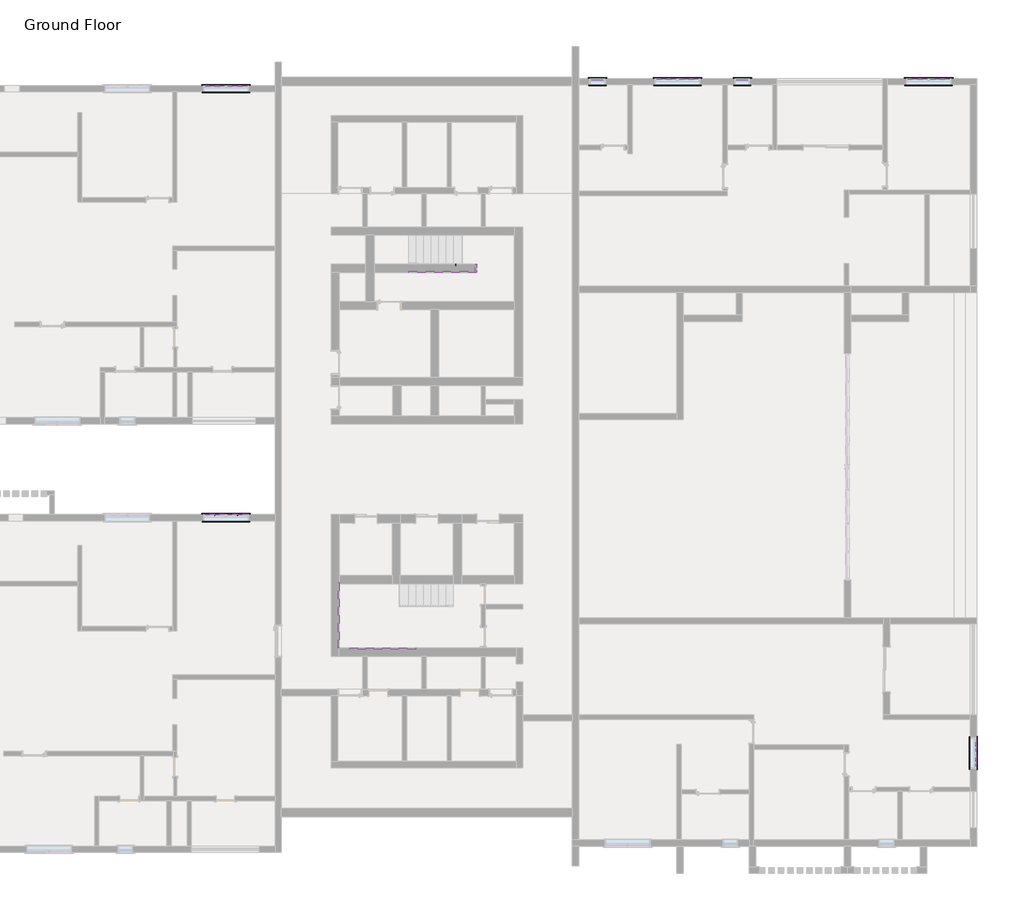
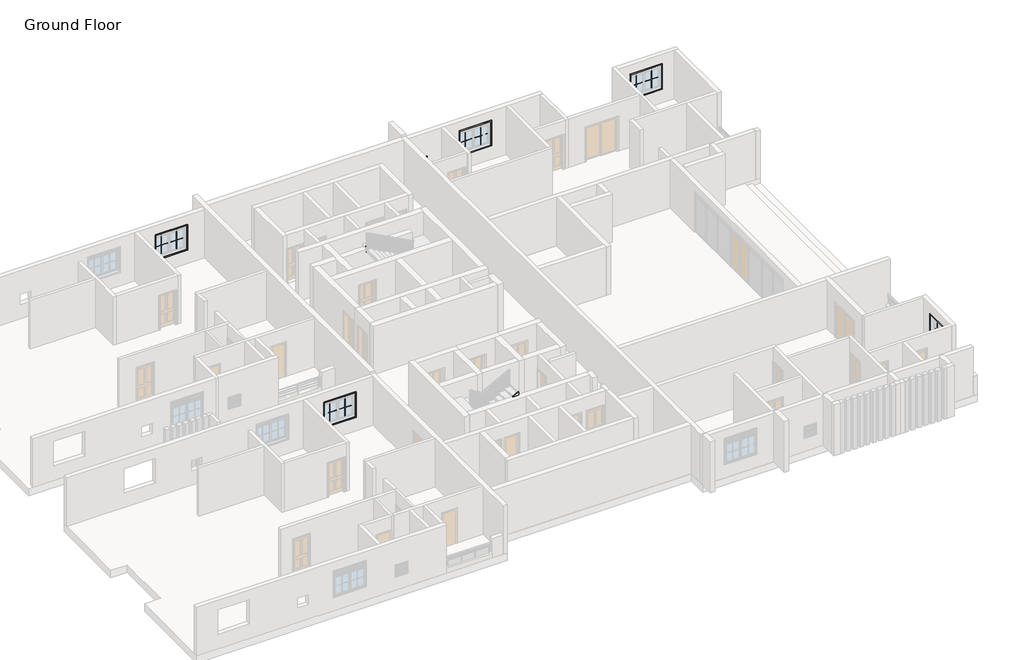
# One storey, part 9 of 9: 38 proxies, 6 members.
"""IFC4 building model written with IfcOpenShell, lengths in millimetres."""

from ifc_helpers import new_model, si_unit, frame, origin, place, context, project, spatial, polyline, outline, extrude, transform, mapped, element, save
from components import muntin_pattern_2x2_muntin_pattern_2x2_dc2504c2, muntin_pattern_2x2_muntin_pattern_2x2_0aa094e9, muntin_pattern_2x2_muntin_pattern_2x2_f17ebf58, muntin_pattern_2x2_muntin_pattern_2x2_cfeb24ad, muntin_pattern_2x2_muntin_pattern_2x2_4dfeb3f3, muntin_pattern_2x2_muntin_pattern_2x2_e852a7e4, muntin_pattern_2x2_muntin_pattern_2x2_3df65231, trim_window_exterior_flat_with_sill_c22f0c79, trim_window_exterior_flat_with_sill_858dc10d, trim_window_exterior_flat_with_sill_92b9b949, trim_window_interior_flat_picture_frame_d1f4d6ef, trim_window_interior_flat_picture_frame_3927330c, trim_window_interior_flat_picture_frame_3bb882cf

model = new_model("IFC4")

# Units and contexts
model_context = context("Model", 3, world=origin())
ifc_project = project(units=[si_unit("LENGTHUNIT", "METRE", prefix="MILLI")], contexts=[model_context])

# Site, building, storey
site = spatial("IfcSite", under=ifc_project)
building = spatial("IfcBuilding", under=site)
storey = spatial("IfcBuildingStorey", under=building, Name="Ground Floor", Elevation=0.0)

# Proxies
placement = place(None, origin())
muntin_pattern_2x2_muntin_pattern_2x2_shape = muntin_pattern_2x2_muntin_pattern_2x2_dc2504c2(model_context)
element("IfcBuildingElementProxy", 1, Name="Muntin Pattern_2x2 : Muntin Pattern_2x2", ObjectType="Muntin Pattern_2x2 : Muntin Pattern_2x2", at=placement, inside=storey, context=model_context, shape_type="MappedRepresentation", body=[
    mapped(muntin_pattern_2x2_muntin_pattern_2x2_shape, transform((1344.6421318, 11632.309892, 984.25), x_axis=(1.0, 0.0, 0.0), y_axis=(0.0, 1.0, 0.0), z_axis=(0.0, 0.0, 1.0))),
])
element("IfcBuildingElementProxy", 2, Name="Muntin Pattern_2x2 : Muntin Pattern_2x2", ObjectType="Muntin Pattern_2x2 : Muntin Pattern_2x2", at=placement, inside=storey, context=model_context, shape_type="MappedRepresentation", body=[
    mapped(muntin_pattern_2x2_muntin_pattern_2x2_shape, transform((1344.6421318, 28955.109892, 984.25), x_axis=(1.0, 0.0, 0.0), y_axis=(0.0, 1.0, 0.0), z_axis=(0.0, 0.0, 1.0))),
])
element("IfcBuildingElementProxy", 3, Name="Muntin Pattern_2x2 : Muntin Pattern_2x2", ObjectType="Muntin Pattern_2x2 : Muntin Pattern_2x2", at=placement, inside=storey, context=model_context, shape_type="MappedRepresentation", body=[
    mapped(muntin_pattern_2x2_muntin_pattern_2x2_shape, transform((19556.4421318, 29234.509892, 984.25), x_axis=(1.0, 0.0, 0.0), y_axis=(0.0, 1.0, 0.0), z_axis=(0.0, 0.0, 1.0))),
])
element("IfcBuildingElementProxy", 4, Name="Muntin Pattern_2x2 : Muntin Pattern_2x2", ObjectType="Muntin Pattern_2x2 : Muntin Pattern_2x2", at=placement, inside=storey, context=model_context, shape_type="MappedRepresentation", body=[
    mapped(muntin_pattern_2x2_muntin_pattern_2x2_shape, transform((29691.0421318, 29234.509892, 984.25), x_axis=(1.0, 0.0, 0.0), y_axis=(0.0, 1.0, 0.0), z_axis=(0.0, 0.0, 1.0))),
])
muntin_pattern_2x2_muntin_pattern_2x2_2_shape = muntin_pattern_2x2_muntin_pattern_2x2_0aa094e9(model_context)
element("IfcBuildingElementProxy", 5, Name="Muntin Pattern_2x2 : Muntin Pattern_2x2", ObjectType="Muntin Pattern_2x2 : Muntin Pattern_2x2", at=placement, inside=storey, context=model_context, shape_type="MappedRepresentation", body=[
    mapped(muntin_pattern_2x2_muntin_pattern_2x2_2_shape, transform((2255.8671318, 11632.309892, 984.25), x_axis=(-1.0, 0.0, 0.0), y_axis=(0.0, -1.0, 0.0), z_axis=(0.0, 0.0, 1.0))),
])
element("IfcBuildingElementProxy", 6, Name="Muntin Pattern_2x2 : Muntin Pattern_2x2", ObjectType="Muntin Pattern_2x2 : Muntin Pattern_2x2", at=placement, inside=storey, context=model_context, shape_type="MappedRepresentation", body=[
    mapped(muntin_pattern_2x2_muntin_pattern_2x2_2_shape, transform((2255.8671318, 28955.109892, 984.25), x_axis=(-1.0, 0.0, 0.0), y_axis=(0.0, -1.0, 0.0), z_axis=(0.0, 0.0, 1.0))),
])
element("IfcBuildingElementProxy", 7, Name="Muntin Pattern_2x2 : Muntin Pattern_2x2", ObjectType="Muntin Pattern_2x2 : Muntin Pattern_2x2", at=placement, inside=storey, context=model_context, shape_type="MappedRepresentation", body=[
    mapped(muntin_pattern_2x2_muntin_pattern_2x2_2_shape, transform((20467.6671318, 29234.509892, 984.25), x_axis=(-1.0, 0.0, 0.0), y_axis=(0.0, -1.0, 0.0), z_axis=(0.0, 0.0, 1.0))),
])
element("IfcBuildingElementProxy", 8, Name="Muntin Pattern_2x2 : Muntin Pattern_2x2", ObjectType="Muntin Pattern_2x2 : Muntin Pattern_2x2", at=placement, inside=storey, context=model_context, shape_type="MappedRepresentation", body=[
    mapped(muntin_pattern_2x2_muntin_pattern_2x2_2_shape, transform((30602.2671318, 29234.509892, 984.25), x_axis=(-1.0, 0.0, 0.0), y_axis=(0.0, -1.0, 0.0), z_axis=(0.0, 0.0, 1.0))),
])
muntin_pattern_2x2_muntin_pattern_2x2_3_shape = muntin_pattern_2x2_muntin_pattern_2x2_f17ebf58(model_context)
element("IfcBuildingElementProxy", 9, Name="Muntin Pattern_2x2 : Muntin Pattern_2x2", ObjectType="Muntin Pattern_2x2 : Muntin Pattern_2x2", at=placement, inside=storey, context=model_context, shape_type="MappedRepresentation", body=[
    mapped(muntin_pattern_2x2_muntin_pattern_2x2_3_shape, transform((2255.8671318, 11632.309892, 2203.45), x_axis=(-1.0, 0.0, 0.0), y_axis=(0.0, -1.0, 0.0), z_axis=(0.0, 0.0, 1.0))),
])
element("IfcBuildingElementProxy", 10, Name="Muntin Pattern_2x2 : Muntin Pattern_2x2", ObjectType="Muntin Pattern_2x2 : Muntin Pattern_2x2", at=placement, inside=storey, context=model_context, shape_type="MappedRepresentation", body=[
    mapped(muntin_pattern_2x2_muntin_pattern_2x2_3_shape, transform((1344.6421318, 11632.309892, 2203.45), x_axis=(-1.0, 0.0, 0.0), y_axis=(0.0, -1.0, 0.0), z_axis=(0.0, 0.0, 1.0))),
])
element("IfcBuildingElementProxy", 11, Name="Muntin Pattern_2x2 : Muntin Pattern_2x2", ObjectType="Muntin Pattern_2x2 : Muntin Pattern_2x2", at=placement, inside=storey, context=model_context, shape_type="MappedRepresentation", body=[
    mapped(muntin_pattern_2x2_muntin_pattern_2x2_3_shape, transform((2255.8671318, 28955.109892, 2203.45), x_axis=(-1.0, 0.0, 0.0), y_axis=(0.0, -1.0, 0.0), z_axis=(0.0, 0.0, 1.0))),
])
element("IfcBuildingElementProxy", 12, Name="Muntin Pattern_2x2 : Muntin Pattern_2x2", ObjectType="Muntin Pattern_2x2 : Muntin Pattern_2x2", at=placement, inside=storey, context=model_context, shape_type="MappedRepresentation", body=[
    mapped(muntin_pattern_2x2_muntin_pattern_2x2_3_shape, transform((1344.6421318, 28955.109892, 2203.45), x_axis=(-1.0, 0.0, 0.0), y_axis=(0.0, -1.0, 0.0), z_axis=(0.0, 0.0, 1.0))),
])
element("IfcBuildingElementProxy", 13, Name="Muntin Pattern_2x2 : Muntin Pattern_2x2", ObjectType="Muntin Pattern_2x2 : Muntin Pattern_2x2", at=placement, inside=storey, context=model_context, shape_type="MappedRepresentation", body=[
    mapped(muntin_pattern_2x2_muntin_pattern_2x2_3_shape, transform((20467.6671318, 29234.509892, 2203.45), x_axis=(-1.0, 0.0, 0.0), y_axis=(0.0, -1.0, 0.0), z_axis=(0.0, 0.0, 1.0))),
])
element("IfcBuildingElementProxy", 14, Name="Muntin Pattern_2x2 : Muntin Pattern_2x2", ObjectType="Muntin Pattern_2x2 : Muntin Pattern_2x2", at=placement, inside=storey, context=model_context, shape_type="MappedRepresentation", body=[
    mapped(muntin_pattern_2x2_muntin_pattern_2x2_3_shape, transform((19556.4421318, 29234.509892, 2203.45), x_axis=(-1.0, 0.0, 0.0), y_axis=(0.0, -1.0, 0.0), z_axis=(0.0, 0.0, 1.0))),
])
element("IfcBuildingElementProxy", 15, Name="Muntin Pattern_2x2 : Muntin Pattern_2x2", ObjectType="Muntin Pattern_2x2 : Muntin Pattern_2x2", at=placement, inside=storey, context=model_context, shape_type="MappedRepresentation", body=[
    mapped(muntin_pattern_2x2_muntin_pattern_2x2_3_shape, transform((30602.2671318, 29234.509892, 2203.45), x_axis=(-1.0, 0.0, 0.0), y_axis=(0.0, -1.0, 0.0), z_axis=(0.0, 0.0, 1.0))),
])
element("IfcBuildingElementProxy", 16, Name="Muntin Pattern_2x2 : Muntin Pattern_2x2", ObjectType="Muntin Pattern_2x2 : Muntin Pattern_2x2", at=placement, inside=storey, context=model_context, shape_type="MappedRepresentation", body=[
    mapped(muntin_pattern_2x2_muntin_pattern_2x2_3_shape, transform((29691.0421318, 29234.509892, 2203.45), x_axis=(-1.0, 0.0, 0.0), y_axis=(0.0, -1.0, 0.0), z_axis=(0.0, 0.0, 1.0))),
])
muntin_pattern_2x2_muntin_pattern_2x2_4_shape = muntin_pattern_2x2_muntin_pattern_2x2_cfeb24ad(model_context)
element("IfcBuildingElementProxy", 17, Name="Muntin Pattern_2x2 : Muntin Pattern_2x2", ObjectType="Muntin Pattern_2x2 : Muntin Pattern_2x2", at=placement, inside=storey, context=model_context, shape_type="MappedRepresentation", body=[
    mapped(muntin_pattern_2x2_muntin_pattern_2x2_4_shape, transform((22628.2546318, 29209.109892, 1241.425), x_axis=(1.0, 0.0, 0.0), y_axis=(0.0, 1.0, 0.0), z_axis=(0.0, 0.0, 1.0))),
])
element("IfcBuildingElementProxy", 18, Name="Muntin Pattern_2x2 : Muntin Pattern_2x2", ObjectType="Muntin Pattern_2x2 : Muntin Pattern_2x2", at=placement, inside=storey, context=model_context, shape_type="MappedRepresentation", body=[
    mapped(muntin_pattern_2x2_muntin_pattern_2x2_4_shape, transform((22628.2546318, 29164.659892, 990.6), x_axis=(1.0, 0.0, 0.0), y_axis=(0.0, 1.0, 0.0), z_axis=(0.0, 0.0, 1.0))),
])
element("IfcBuildingElementProxy", 19, Name="Muntin Pattern_2x2 : Muntin Pattern_2x2", ObjectType="Muntin Pattern_2x2 : Muntin Pattern_2x2", at=placement, inside=storey, context=model_context, shape_type="MappedRepresentation", body=[
    mapped(muntin_pattern_2x2_muntin_pattern_2x2_4_shape, transform((16786.2546318, 29209.109892, 1241.425), x_axis=(1.0, 0.0, 0.0), y_axis=(0.0, 1.0, 0.0), z_axis=(0.0, 0.0, 1.0))),
])
element("IfcBuildingElementProxy", 20, Name="Muntin Pattern_2x2 : Muntin Pattern_2x2", ObjectType="Muntin Pattern_2x2 : Muntin Pattern_2x2", at=placement, inside=storey, context=model_context, shape_type="MappedRepresentation", body=[
    mapped(muntin_pattern_2x2_muntin_pattern_2x2_4_shape, transform((16786.2546318, 29164.659892, 990.6), x_axis=(1.0, 0.0, 0.0), y_axis=(0.0, 1.0, 0.0), z_axis=(0.0, 0.0, 1.0))),
])
muntin_pattern_2x2_muntin_pattern_2x2_5_shape = muntin_pattern_2x2_muntin_pattern_2x2_4dfeb3f3(model_context)
element("IfcBuildingElementProxy", 21, Name="Muntin Pattern_2x2 : Muntin Pattern_2x2", ObjectType="Muntin Pattern_2x2 : Muntin Pattern_2x2", at=placement, inside=storey, context=model_context, shape_type="MappedRepresentation", body=[
    mapped(muntin_pattern_2x2_muntin_pattern_2x2_5_shape, transform((32067.5296318, 2318.447392, 984.25), x_axis=(0.0, -1.0, 0.0), y_axis=(1.0, 0.0, 0.0), z_axis=(0.0, 0.0, 1.0))),
])
muntin_pattern_2x2_muntin_pattern_2x2_6_shape = muntin_pattern_2x2_muntin_pattern_2x2_e852a7e4(model_context)
element("IfcBuildingElementProxy", 22, Name="Muntin Pattern_2x2 : Muntin Pattern_2x2", ObjectType="Muntin Pattern_2x2 : Muntin Pattern_2x2", at=placement, inside=storey, context=model_context, shape_type="MappedRepresentation", body=[
    mapped(muntin_pattern_2x2_muntin_pattern_2x2_6_shape, transform((32067.5296318, 1712.022392, 984.25), x_axis=(0.0, 1.0, 0.0), y_axis=(-1.0, 0.0, 0.0), z_axis=(0.0, 0.0, 1.0))),
])
muntin_pattern_2x2_muntin_pattern_2x2_7_shape = muntin_pattern_2x2_muntin_pattern_2x2_3df65231(model_context)
element("IfcBuildingElementProxy", 23, Name="Muntin Pattern_2x2 : Muntin Pattern_2x2", ObjectType="Muntin Pattern_2x2 : Muntin Pattern_2x2", at=placement, inside=storey, context=model_context, shape_type="MappedRepresentation", body=[
    mapped(muntin_pattern_2x2_muntin_pattern_2x2_7_shape, transform((32067.5296318, 1712.022392, 2203.45), x_axis=(0.0, 1.0, 0.0), y_axis=(-1.0, 0.0, 0.0), z_axis=(0.0, 0.0, 1.0))),
])
element("IfcBuildingElementProxy", 24, Name="Muntin Pattern_2x2 : Muntin Pattern_2x2", ObjectType="Muntin Pattern_2x2 : Muntin Pattern_2x2", at=placement, inside=storey, context=model_context, shape_type="MappedRepresentation", body=[
    mapped(muntin_pattern_2x2_muntin_pattern_2x2_7_shape, transform((32067.5296318, 2318.447392, 2203.45), x_axis=(0.0, 1.0, 0.0), y_axis=(-1.0, 0.0, 0.0), z_axis=(0.0, 0.0, 1.0))),
])
trim_window_exterior_flat_with_sill_shape = trim_window_exterior_flat_with_sill_c22f0c79(model_context)
element("IfcBuildingElementProxy", 25, Name="Trim-Window-Exterior-Flat : with Sill", ObjectType="Trim-Window-Exterior-Flat : with Sill", at=placement, inside=storey, context=model_context, shape_type="MappedRepresentation", body=[
    mapped(trim_window_exterior_flat_with_sill_shape, transform((1800.2546318, 11641.834892, 2438.4), x_axis=(-1.0, 0.0, 0.0), y_axis=(0.0, 0.0, 1.0), z_axis=(0.0, 1.0, 0.0))),
])
element("IfcBuildingElementProxy", 26, Name="Trim-Window-Exterior-Flat : with Sill", ObjectType="Trim-Window-Exterior-Flat : with Sill", at=placement, inside=storey, context=model_context, shape_type="MappedRepresentation", body=[
    mapped(trim_window_exterior_flat_with_sill_shape, transform((1800.2546318, 28964.634892, 2438.4), x_axis=(-1.0, 0.0, 0.0), y_axis=(0.0, 0.0, 1.0), z_axis=(0.0, 1.0, 0.0))),
])
element("IfcBuildingElementProxy", 27, Name="Trim-Window-Exterior-Flat : with Sill", ObjectType="Trim-Window-Exterior-Flat : with Sill", at=placement, inside=storey, context=model_context, shape_type="MappedRepresentation", body=[
    mapped(trim_window_exterior_flat_with_sill_shape, transform((20012.0546318, 29244.034892, 2438.4), x_axis=(-1.0, 0.0, 0.0), y_axis=(0.0, 0.0, 1.0), z_axis=(0.0, 1.0, 0.0))),
])
element("IfcBuildingElementProxy", 28, Name="Trim-Window-Exterior-Flat : with Sill", ObjectType="Trim-Window-Exterior-Flat : with Sill", at=placement, inside=storey, context=model_context, shape_type="MappedRepresentation", body=[
    mapped(trim_window_exterior_flat_with_sill_shape, transform((30146.6546318, 29244.034892, 2438.4), x_axis=(-1.0, 0.0, 0.0), y_axis=(0.0, 0.0, 1.0), z_axis=(0.0, 1.0, 0.0))),
])
trim_window_exterior_flat_with_sill_2_shape = trim_window_exterior_flat_with_sill_858dc10d(model_context)
element("IfcBuildingElementProxy", 29, Name="Trim-Window-Exterior-Flat : with Sill", ObjectType="Trim-Window-Exterior-Flat : with Sill", at=placement, inside=storey, context=model_context, shape_type="MappedRepresentation", body=[
    mapped(trim_window_exterior_flat_with_sill_2_shape, transform((22628.2546318, 29244.034892, 1524.0), x_axis=(-1.0, 0.0, 0.0), y_axis=(0.0, 0.0, 1.0), z_axis=(0.0, 1.0, 0.0))),
])
element("IfcBuildingElementProxy", 30, Name="Trim-Window-Exterior-Flat : with Sill", ObjectType="Trim-Window-Exterior-Flat : with Sill", at=placement, inside=storey, context=model_context, shape_type="MappedRepresentation", body=[
    mapped(trim_window_exterior_flat_with_sill_2_shape, transform((16786.2546318, 29244.034892, 1524.0), x_axis=(-1.0, 0.0, 0.0), y_axis=(0.0, 0.0, 1.0), z_axis=(0.0, 1.0, 0.0))),
])
trim_window_exterior_flat_with_sill_3_shape = trim_window_exterior_flat_with_sill_92b9b949(model_context)
element("IfcBuildingElementProxy", 31, Name="Trim-Window-Exterior-Flat : with Sill", ObjectType="Trim-Window-Exterior-Flat : with Sill", at=placement, inside=storey, context=model_context, shape_type="MappedRepresentation", body=[
    mapped(trim_window_exterior_flat_with_sill_3_shape, transform((32077.0546318, 2015.234892, 2438.4), x_axis=(0.0, 1.0, 0.0), y_axis=(0.0, 0.0, 1.0), z_axis=(1.0, 0.0, 0.0))),
])
trim_window_interior_flat_picture_frame_shape = trim_window_interior_flat_picture_frame_d1f4d6ef(model_context)
element("IfcBuildingElementProxy", 32, Name="Trim-Window-Interior-Flat : Picture Frame", ObjectType="Trim-Window-Interior-Flat : Picture Frame", at=placement, inside=storey, context=model_context, shape_type="MappedRepresentation", body=[
    mapped(trim_window_interior_flat_picture_frame_shape, transform((1800.2546318, 11387.834892, 2438.4), x_axis=(1.0, 0.0, 0.0), y_axis=(0.0, 0.0, 1.0), z_axis=(0.0, -1.0, 0.0))),
])
element("IfcBuildingElementProxy", 33, Name="Trim-Window-Interior-Flat : Picture Frame", ObjectType="Trim-Window-Interior-Flat : Picture Frame", at=placement, inside=storey, context=model_context, shape_type="MappedRepresentation", body=[
    mapped(trim_window_interior_flat_picture_frame_shape, transform((1800.2546318, 28710.634892, 2438.4), x_axis=(1.0, 0.0, 0.0), y_axis=(0.0, 0.0, 1.0), z_axis=(0.0, -1.0, 0.0))),
])
element("IfcBuildingElementProxy", 34, Name="Trim-Window-Interior-Flat : Picture Frame", ObjectType="Trim-Window-Interior-Flat : Picture Frame", at=placement, inside=storey, context=model_context, shape_type="MappedRepresentation", body=[
    mapped(trim_window_interior_flat_picture_frame_shape, transform((20012.0546318, 28990.034892, 2438.4), x_axis=(1.0, 0.0, 0.0), y_axis=(0.0, 0.0, 1.0), z_axis=(0.0, -1.0, 0.0))),
])
element("IfcBuildingElementProxy", 35, Name="Trim-Window-Interior-Flat : Picture Frame", ObjectType="Trim-Window-Interior-Flat : Picture Frame", at=placement, inside=storey, context=model_context, shape_type="MappedRepresentation", body=[
    mapped(trim_window_interior_flat_picture_frame_shape, transform((30146.6546318, 28990.034892, 2438.4), x_axis=(1.0, 0.0, 0.0), y_axis=(0.0, 0.0, 1.0), z_axis=(0.0, -1.0, 0.0))),
])
trim_window_interior_flat_picture_frame_2_shape = trim_window_interior_flat_picture_frame_3927330c(model_context)
element("IfcBuildingElementProxy", 36, Name="Trim-Window-Interior-Flat : Picture Frame", ObjectType="Trim-Window-Interior-Flat : Picture Frame", at=placement, inside=storey, context=model_context, shape_type="MappedRepresentation", body=[
    mapped(trim_window_interior_flat_picture_frame_2_shape, transform((22628.2546318, 28990.034892, 1524.0), x_axis=(1.0, 0.0, 0.0), y_axis=(0.0, 0.0, 1.0), z_axis=(0.0, -1.0, 0.0))),
])
element("IfcBuildingElementProxy", 37, Name="Trim-Window-Interior-Flat : Picture Frame", ObjectType="Trim-Window-Interior-Flat : Picture Frame", at=placement, inside=storey, context=model_context, shape_type="MappedRepresentation", body=[
    mapped(trim_window_interior_flat_picture_frame_2_shape, transform((16786.2546318, 28990.034892, 1524.0), x_axis=(1.0, 0.0, 0.0), y_axis=(0.0, 0.0, 1.0), z_axis=(0.0, -1.0, 0.0))),
])
trim_window_interior_flat_picture_frame_3_shape = trim_window_interior_flat_picture_frame_3bb882cf(model_context)
element("IfcBuildingElementProxy", 38, Name="Trim-Window-Interior-Flat : Picture Frame", ObjectType="Trim-Window-Interior-Flat : Picture Frame", at=placement, inside=storey, context=model_context, shape_type="MappedRepresentation", body=[
    mapped(trim_window_interior_flat_picture_frame_3_shape, transform((31823.0546318, 2015.234892, 2438.4), x_axis=(0.0, -1.0, 0.0), y_axis=(0.0, 0.0, 1.0), z_axis=(-1.0, 0.0, 0.0))),
])

# Members
element("IfcMember", 39, ObjectType="Stringer - 2\" Width", at=placement, inside=storey, context=model_context, shape_type="SweptSolid", body=[
    extrude(outline(polyline([(0.0, 10969.6546318), (208.3550016, 10969.6546318), (2097.5052632, 7522.7050673), (2097.5052632, 6888.51765), (0.0, 10715.6324119), (0.0, 10969.6546318)])), frame((0.0, 8847.834892, 0.0), z_axis=(0.0, 1.0, 0.0), x_axis=(0.0, 0.0, 1.0)), (0.0, 0.0, 1.0), 50.8),
])
element("IfcMember", 40, ObjectType="Stringer - 2\" Width", at=placement, inside=storey, context=model_context, shape_type="SweptSolid", body=[
    extrude(outline(polyline([(6321.4546318, 8898.634892), (6372.2546318, 8898.634892), (6372.2546318, 6257.034892), (6321.4546318, 6257.034892), (6321.4546318, 8898.634892)])), frame((0.0, 0.0, 1792.7052632), z_axis=(0.0, 0.0, 1.0), x_axis=(1.0, 0.0, 0.0)), (0.0, 0.0, 1.0), 304.8),
])
element("IfcMember", 41, ObjectType="Stringer - 2\" Width", at=placement, inside=storey, context=model_context, shape_type="SweptSolid", body=[
    extrude(outline(polyline([(1792.7052632, 7429.0719482), (2888.8632361, 9445.6546318), (3235.7827571, 9445.6546318), (1792.7052632, 6790.8501628), (1792.7052632, 7429.0719482)])), frame((0.0, 6206.234892, 0.0), z_axis=(0.0, 1.0, 0.0), x_axis=(0.0, 0.0, 1.0)), (0.0, 0.0, 1.0), 50.8),
])
element("IfcMember", 42, ObjectType="Stringer - 2\" Width", at=placement, inside=storey, context=model_context, shape_type="SweptSolid", body=[
    extrude(outline(polyline([(205.0640844, 9166.2546318), (0.0, 9166.2546318), (0.0, 9431.3744736), (1274.3220831, 11858.6546318), (1618.5740844, 11858.6546318), (205.0640844, 9166.2546318)])), frame((0.0, 21700.234892, 0.0), z_axis=(0.0, 1.0, 0.0), x_axis=(0.0, 0.0, 1.0)), (0.0, 0.0, 1.0), 50.8),
])
element("IfcMember", 43, ObjectType="Stringer - 2\" Width", at=placement, inside=storey, context=model_context, shape_type="SweptSolid", body=[
    extrude(outline(polyline([(11858.6546318, 21751.034892), (11909.4546318, 21751.034892), (11909.4546318, 21471.634892), (11858.6546318, 21471.634892), (11858.6546318, 21751.034892)])), frame((0.0, 0.0, 1371.6), z_axis=(0.0, 0.0, 1.0), x_axis=(1.0, 0.0, 0.0)), (0.0, 0.0, 1.0), 304.8),
])
element("IfcMember", 44, ObjectType="Stringer - 2\" Width", at=placement, inside=storey, context=model_context, shape_type="SweptSolid", body=[
    extrude(outline(polyline([(1461.0120831, 11909.4546318), (1805.2640844, 11909.4546318), (3245.4440844, 9166.2546318), (2901.1920831, 9166.2546318), (1461.0120831, 11909.4546318)])), frame((0.0, 21420.834892, 0.0), z_axis=(0.0, 1.0, 0.0), x_axis=(0.0, 0.0, 1.0)), (0.0, 0.0, 1.0), 50.8),
])

save(model, "model.ifc")

# Revit data of these elements
# Type "Muntin Pattern_2x2 : Muntin Pattern_2x2"
#   Width [instance default] = 4' - 0"
#   Thickness = 0' - 0 1/2"
#   Height [instance default] = 4' - 0"
#   Distance = 0' - 0 3/4"
#   Interior Material [instance default] = none
#   Exterior Material [instance default] = none
#   Default Elevation = 0
# Type "Trim-Window-Exterior-Flat : with Sill"
#   Trim Width = 0' - 2 1/4"
#   Trim Thickness_Picture Frame = 0' - 1 1/4"
#   Trim Thickness_with Sill = 0' - 0 3/4"
#   Sill Thickness = 0' - 1 1/4"
#   Opening Width [instance default] = 2' - 0"
#   Opening Height [instance default] = 3' - 0"
#   Default Elevation = 4' - 0"
#   Sill = yes
#   Picture Frame = no
#   Trim Material [instance default] = none
# Type "Trim-Window-Interior-Flat : Picture Frame"
#   Trim Thickness_Picture Frame = 0' - 1 1/4"
#   Trim Width = 0' - 2 1/4"
#   Trim Thickness_with Sill = 0' - 0 3/4"
#   Sill Thickness = 0' - 1 1/4"
#   Opening Width [instance default] = 2' - 0"
#   Opening Height [instance default] = 3' - 0"
#   Default Elevation = 4' - 0"
#   Sill = no
#   Picture Frame = yes
#   Trim Material [instance default] = none
# Elements 1, 2, 3, 4, 5, 6, 7, 8 (IfcBuildingElementProxy, "Muntin Pattern_2x2 : Muntin Pattern_2x2")
#   Width = 2' - 6 5/8"
#   Height = 3' - 6 1/2"
#   Interior Material = Wood - Stained
#   Exterior Material = Clad - White
#   Phase Created = New Construction
#   Materials on its faces: "Clad - White", "Wood - Stained"
# Elements 9, 10, 11, 12, 13, 14, 15, 16 (IfcBuildingElementProxy, "Muntin Pattern_2x2 : Muntin Pattern_2x2")
#   Width = 2' - 6 5/8"
#   Height = 0' - 6 1/2"
#   Interior Material = Wood - Stained
#   Exterior Material = Clad - White
#   Phase Created = New Construction
#   Materials on its faces: "Clad - White", "Wood - Stained"
# Elements 17, 18, 19, 20 (IfcBuildingElementProxy, "Muntin Pattern_2x2 : Muntin Pattern_2x2")
#   Width = 1' - 6"
#   Height = 0' - 8 1/8"
#   Interior Material = Wood - Stained
#   Exterior Material = Clad - White
#   Phase Created = New Construction
#   Materials on its faces: "Clad - White", "Wood - Stained"
# Elements 21, 22 (IfcBuildingElementProxy, "Muntin Pattern_2x2 : Muntin Pattern_2x2")
#   Width = 1' - 6 5/8"
#   Height = 3' - 6 1/2"
#   Interior Material = Wood - Stained
#   Exterior Material = Clad - White
#   Phase Created = New Construction
#   Materials on its faces: "Clad - White", "Wood - Stained"
# Elements 23, 24 (IfcBuildingElementProxy, "Muntin Pattern_2x2 : Muntin Pattern_2x2")
#   Width = 1' - 6 5/8"
#   Height = 0' - 6 1/2"
#   Interior Material = Wood - Stained
#   Exterior Material = Clad - White
#   Phase Created = New Construction
#   Materials on its faces: "Clad - White", "Wood - Stained"
# Elements 25, 26, 27, 28 (IfcBuildingElementProxy, "Trim-Window-Exterior-Flat : with Sill")
#   Opening Width = 6' - 0"
#   Opening Height = 5' - 0"
#   Trim Material = Clad - White
#   Phase Created = New Construction
#   Materials on its faces: "Clad - White"
# Elements 29, 30 (IfcBuildingElementProxy, "Trim-Window-Exterior-Flat : with Sill")
#   Opening Width = 2' - 0"
#   Opening Height = 2' - 0"
#   Trim Material = Clad - White
#   Phase Created = New Construction
#   Materials on its faces: "Clad - White"
# Element 31 (IfcBuildingElementProxy, "Trim-Window-Exterior-Flat : with Sill")
#   Opening Width = 4' - 0"
#   Opening Height = 5' - 0"
#   Trim Material = Clad - White
#   Phase Created = New Construction
#   Materials on its faces: "Clad - White"
# Elements 32, 33, 34, 35 (IfcBuildingElementProxy, "Trim-Window-Interior-Flat : Picture Frame")
#   Opening Width = 6' - 0"
#   Opening Height = 5' - 0"
#   Trim Material = Wood - Stained
#   Phase Created = New Construction
#   Materials on its faces: "Wood - Stained"
# Elements 36, 37 (IfcBuildingElementProxy, "Trim-Window-Interior-Flat : Picture Frame")
#   Opening Width = 2' - 0"
#   Opening Height = 2' - 0"
#   Trim Material = Wood - Stained
#   Phase Created = New Construction
#   Materials on its faces: "Wood - Stained"
# Element 38 (IfcBuildingElementProxy, "Trim-Window-Interior-Flat : Picture Frame")
#   Opening Width = 4' - 0"
#   Opening Height = 5' - 0"
#   Trim Material = Wood - Stained
#   Phase Created = New Construction
#   Materials on its faces: "Wood - Stained"
# Elements 39, 40, 41, 42, 43, 44 (IfcMember, "Stringer - 2\" Width")
#   Phase Created = New Construction
# Materials
#   "Clad - White": class "Wood", colour RGB 242 242 238, transparency 0, Cost = 0
#   "Wood - Stained": class "Wood", colour RGB 224 178 126, transparency 0, Cost = 0
